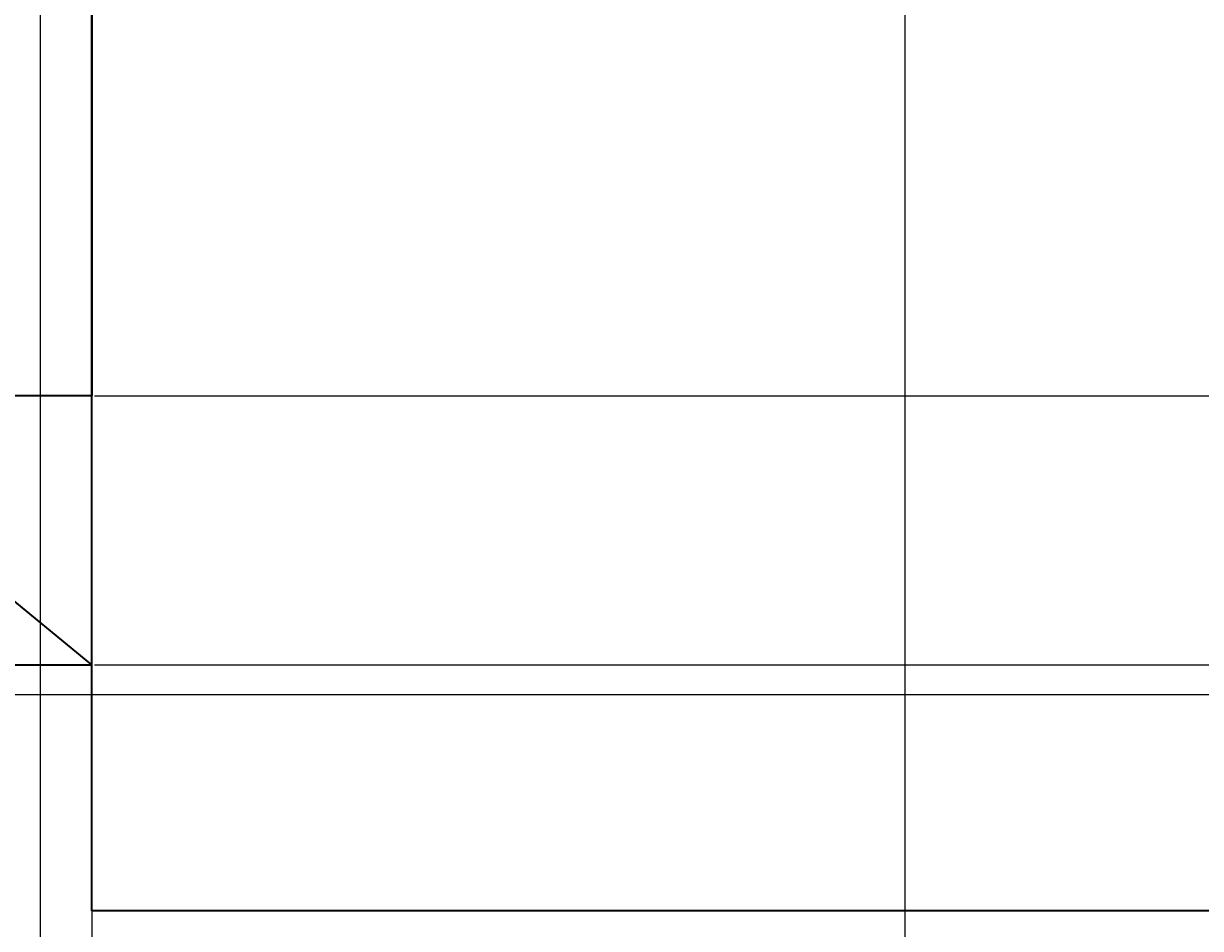
# Model space of a CAD drawing. Units: inches. Extents: x 27 to 200, y -50 to 102.
# Tile 22 of 26: x 145 to 172, y 39 to 61. Entities that reach past the tile are written whole.
import ezdxf

# ---------------------------------------------------------------- set-up
doc = ezdxf.new("R2010")
doc.units = ezdxf.units.IN
doc.header["$MEASUREMENT"] = 0
doc.layers.add('A-ANNO-DIMS', color=2, linetype='Continuous', lineweight=18)
doc.layers.add('A-ELEV', color=7, linetype='Continuous', lineweight=35)
doc.styles.get("Standard").update_dxf_attribs({"font": 'arial.ttf'})
doc.dimstyles.get("Standard").update_dxf_attribs({"dimtxt": 0.18, "dimasz": 0.18, "dimexe": 0.18, "dimexo": 0.0625, "dimgap": 0.09, "dimtad": 0, "dimtih": 1, "dimtoh": 1, "dimdec": 4, "dimzin": 0, "dimdsep": 46, "dimtxsty": 'Standard', "dimcen": 0.09, "dimadec": 0, "dimazin": 0, "dimtfac": 1, "dimtdec": 4, "dimtofl": 0, "dimtmove": 0, "dimatfit": 3, "dimfxl": 1, "dimtolj": 1, "dimtzin": 0, "dimarcsym": 0})

# ---------------------------------------------------------------- blocks, each defined once
blk = doc.blocks.new('*D28')
at = {"layer": 'A-ANNO-DIMS', "color": 0, "lineweight": -2, "transparency": 16777216}
for p, q in [((146.479, 51.926), (199.797, 51.926)), ((199.617, 51.746), (199.617, 46.073)), ((199.617, 40.036), (199.617, 45.709)), ((146.479, 39.856), (199.797, 39.856))]:
    blk.add_line(p, q, dxfattribs=at)
at = {"layer": 'A-ANNO-DIMS', "color": 0, "transparency": 16777216}
for points in [[(199.587, 51.746), (199.647, 51.746), (199.617, 51.926)], [(199.587, 40.036), (199.647, 40.036), (199.617, 39.856)]]:
    blk.add_solid(points, dxfattribs=at)
at = {"layer": 'Defpoints', "color": 0, "transparency": 16777216}
for p in [(146.417, 51.926), (199.617, 51.926), (146.417, 39.856)]:
    blk.add_point(p, dxfattribs=at)
at = {"layer": 'A-ANNO-DIMS', "color": 0, "transparency": 16777216, "insert": (199.617, 45.891), "char_height": 0.18, "attachment_point": 5}
blk.add_mtext('\\A1;12.07', dxfattribs=at)
blk = doc.blocks.new('*D29')
at = {"layer": 'A-ANNO-DIMS', "color": 0, "lineweight": -2, "transparency": 16777216}
for p, q in [((146.479, 65.587), (199.797, 65.587)), ((199.617, 65.407), (199.617, 58.938)), ((199.617, 52.106), (199.617, 58.575)), ((146.479, 51.926), (199.797, 51.926))]:
    blk.add_line(p, q, dxfattribs=at)
at = {"layer": 'A-ANNO-DIMS', "color": 0, "transparency": 16777216}
for points in [[(199.587, 65.407), (199.647, 65.407), (199.617, 65.587)], [(199.587, 52.106), (199.647, 52.106), (199.617, 51.926)]]:
    blk.add_solid(points, dxfattribs=at)
at = {"layer": 'Defpoints', "color": 0, "transparency": 16777216}
for p in [(146.417, 65.587), (199.617, 65.587), (146.417, 51.926)]:
    blk.add_point(p, dxfattribs=at)
at = {"layer": 'A-ANNO-DIMS', "color": 0, "transparency": 16777216, "insert": (199.617, 58.756), "char_height": 0.18, "attachment_point": 5}
blk.add_mtext('\\A1;13.66', dxfattribs=at)
blk = doc.blocks.new('*D48')
at = {"layer": 'A-ANNO-DIMS', "color": 0, "lineweight": -2, "transparency": 16777216}
for p, q in [((84.479, 44.926), (199.797, 44.926)), ((199.617, 44.746), (199.617, 14.26)), ((199.617, -16.589), (199.617, 13.897)), ((84.479, -16.769), (199.797, -16.769))]:
    blk.add_line(p, q, dxfattribs=at)
at = {"layer": 'A-ANNO-DIMS', "color": 0, "transparency": 16777216}
for points in [[(199.587, 44.746), (199.647, 44.746), (199.617, 44.926)], [(199.587, -16.589), (199.647, -16.589), (199.617, -16.769)]]:
    blk.add_solid(points, dxfattribs=at)
at = {"layer": 'Defpoints', "color": 0, "transparency": 16777216}
for p in [(84.417, 44.926), (199.617, 44.926), (84.417, -16.769)]:
    blk.add_point(p, dxfattribs=at)
at = {"layer": 'A-ANNO-DIMS', "color": 0, "transparency": 16777216, "insert": (199.617, 14.079), "char_height": 0.18, "attachment_point": 5}
blk.add_mtext('\\A1;61.7', dxfattribs=at)
blk = doc.blocks.new('*D50')
at = {"layer": 'A-ANNO-DIMS', "color": 0, "lineweight": -2, "transparency": 16777216}
for p, q in [((138.722, 51.989), (138.722, 102.306)), ((138.902, 102.126), (142.176, 102.126)), ((146.237, 102.126), (142.963, 102.126)), ((146.417, 51.989), (146.417, 102.306))]:
    blk.add_line(p, q, dxfattribs=at)
at = {"layer": 'A-ANNO-DIMS', "color": 0, "transparency": 16777216}
for points in [[(138.902, 102.156), (138.902, 102.096), (138.722, 102.126)], [(146.237, 102.156), (146.237, 102.096), (146.417, 102.126)]]:
    blk.add_solid(points, dxfattribs=at)
at = {"layer": 'Defpoints', "color": 0, "transparency": 16777216}
for p in [(146.417, 102.126), (138.722, 51.926), (146.417, 51.926)]:
    blk.add_point(p, dxfattribs=at)
at = {"layer": 'A-ANNO-DIMS', "color": 0, "transparency": 16777216, "insert": (142.569, 102.126), "char_height": 0.18, "attachment_point": 5}
blk.add_mtext('\\A1;7.695', dxfattribs=at)
blk = doc.blocks.new('*D51')
at = {"layer": 'A-ANNO-DIMS', "color": 0, "lineweight": -2, "transparency": 16777216}
for p, q in [((120.417, 45.561), (120.417, -25.149)), ((146.417, 45.561), (146.417, -25.149)), ((120.597, -24.969), (133.197, -24.969)), ((146.237, -24.969), (133.637, -24.969))]:
    blk.add_line(p, q, dxfattribs=at)
at = {"layer": 'A-ANNO-DIMS', "color": 0, "transparency": 16777216}
for points in [[(120.597, -24.939), (120.597, -24.999), (120.417, -24.969)], [(146.237, -24.939), (146.237, -24.999), (146.417, -24.969)]]:
    blk.add_solid(points, dxfattribs=at)
at = {"layer": 'Defpoints', "color": 0, "transparency": 16777216}
for p in [(120.417, 45.623), (146.417, 45.623), (146.417, -24.969)]:
    blk.add_point(p, dxfattribs=at)
at = {"layer": 'A-ANNO-DIMS', "color": 0, "transparency": 16777216, "insert": (133.417, -24.969), "char_height": 0.18, "attachment_point": 5}
blk.add_mtext('\\A1;26', dxfattribs=at)
blk = doc.blocks.new('*D52')
at = {"layer": 'A-ANNO-DIMS', "color": 0, "lineweight": -2, "transparency": 16777216}
for p, q in [((146.479, 51.926), (199.797, 51.926)), ((199.617, 51.746), (199.617, 48.957)), ((199.617, 45.803), (199.617, 48.593)), ((146.479, 45.623), (199.797, 45.623))]:
    blk.add_line(p, q, dxfattribs=at)
at = {"layer": 'A-ANNO-DIMS', "color": 0, "transparency": 16777216}
for points in [[(199.587, 51.746), (199.647, 51.746), (199.617, 51.926)], [(199.587, 45.803), (199.647, 45.803), (199.617, 45.623)]]:
    blk.add_solid(points, dxfattribs=at)
at = {"layer": 'Defpoints', "color": 0, "transparency": 16777216}
for p in [(146.417, 51.926), (199.617, 51.926), (146.417, 45.623)]:
    blk.add_point(p, dxfattribs=at)
at = {"layer": 'A-ANNO-DIMS', "color": 0, "transparency": 16777216, "insert": (199.617, 48.775), "char_height": 0.18, "attachment_point": 5}
blk.add_mtext('\\A1;6.303', dxfattribs=at)
blk = doc.blocks.new('*D64')
at = {"layer": 'A-ANNO-DIMS', "color": 0, "lineweight": -2, "transparency": 16777216}
for p, q in [((145.216, 13.517), (145.216, 102.306)), ((145.396, 102.126), (154.884, 102.126)), ((165.303, 102.126), (155.815, 102.126)), ((165.483, 13.517), (165.483, 102.306))]:
    blk.add_line(p, q, dxfattribs=at)
at = {"layer": 'A-ANNO-DIMS', "color": 0, "transparency": 16777216}
for points in [[(145.396, 102.156), (145.396, 102.096), (145.216, 102.126)], [(165.303, 102.156), (165.303, 102.096), (165.483, 102.126)]]:
    blk.add_solid(points, dxfattribs=at)
at = {"layer": 'Defpoints', "color": 0, "transparency": 16777216}
for p in [(165.483, 102.126), (145.216, 13.455), (165.483, 13.455)]:
    blk.add_point(p, dxfattribs=at)
at = {"layer": 'A-ANNO-DIMS', "color": 0, "transparency": 16777216, "insert": (155.35, 102.126), "char_height": 0.18, "attachment_point": 5}
blk.add_mtext('\\A1;20.267', dxfattribs=at)

msp = doc.modelspace()

# ---------------------------------------------------------------- linework, layer by layer
at = {"layer": 'A-ELEV'}
for p, q in [((146.4169, 87.9264), (146.4169, 51.9264)), ((146.4169, 39.8559), (146.4169, 65.5865)), ((146.4169, 51.9264), (120.4169, 51.9264)), ((146.4169, 45.6231), (138.7218, 51.9264)), ((120.4169, 45.6231), (146.4169, 45.6231)), ((182.4169, 39.8559), (146.4169, 39.8559))]:
    msp.add_line(p, q, dxfattribs=at)

# ---------------------------------------------------------------- dimensions: what is measured, and where the dimension line sits
at = {"layer": 'A-ANNO-DIMS'}
for base, p1, p2, override, picture, middle in [((146.4169, 102.1264), (138.7218, 51.9264), (146.4169, 51.9264), {"dimdec": 3, "dimlfac": 1, "dimrnd": 0, "dimzin": 0, "dimdsep": 46, "dimlunit": 2}, '*D50', (142.5694, 102.1264)), ((165.4832, 102.1264), (145.216, 13.4548), (165.4832, 13.4548), {"dimdec": 3, "dimlfac": 1, "dimrnd": 0, "dimzin": 0, "dimdsep": 46, "dimlunit": 2}, '*D64', (155.3496, 102.1264)), ((146.4169, -24.9693), (120.4169, 45.6231), (146.4169, 45.6231), {"dimdec": 0, "dimlfac": 1, "dimrnd": 0, "dimzin": 0, "dimdsep": 46, "dimlunit": 2}, '*D51', (133.4169, -24.9693))]:
    dim = msp.add_linear_dim(base=base, p1=p1, p2=p2, dimstyle='Standard', override=override, dxfattribs=at)
    dim.commit()
    dim.dimension.update_dxf_attribs({"geometry": picture, "text_midpoint": middle})
for base, p1, p2, override, picture, middle in [((199.6169, 65.5865), (146.4169, 51.9264), (146.4169, 65.5865), {"dimdec": 2, "dimlfac": 1, "dimrnd": 0, "dimzin": 0, "dimdsep": 46, "dimlunit": 2}, '*D29', (199.6169, 58.7565)), ((199.6169, 51.9264), (146.4169, 39.8559), (146.4169, 51.9264), {"dimdec": 2, "dimlfac": 1, "dimrnd": 0, "dimzin": 0, "dimdsep": 46, "dimlunit": 2}, '*D28', (199.6169, 45.8912)), ((199.6169, 51.9264), (146.4169, 45.6231), (146.4169, 51.9264), {"dimdec": 3, "dimlfac": 1, "dimrnd": 0, "dimzin": 0, "dimdsep": 46, "dimlunit": 2}, '*D52', (199.6169, 48.7748)), ((199.6169, 44.9264), (84.4169, -16.7693), (84.4169, 44.9264), {"dimdec": 1, "dimlfac": 1, "dimrnd": 0, "dimzin": 0, "dimdsep": 46, "dimlunit": 2}, '*D48', (199.6169, 14.0786))]:
    dim = msp.add_linear_dim(base=base, p1=p1, p2=p2, angle=90, dimstyle='Standard', override=override, dxfattribs=at)
    dim.commit()
    dim.dimension.update_dxf_attribs({"geometry": picture, "text_midpoint": middle})

doc.saveas('drawing.dxf')
